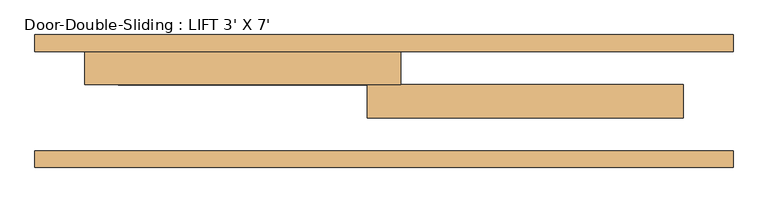
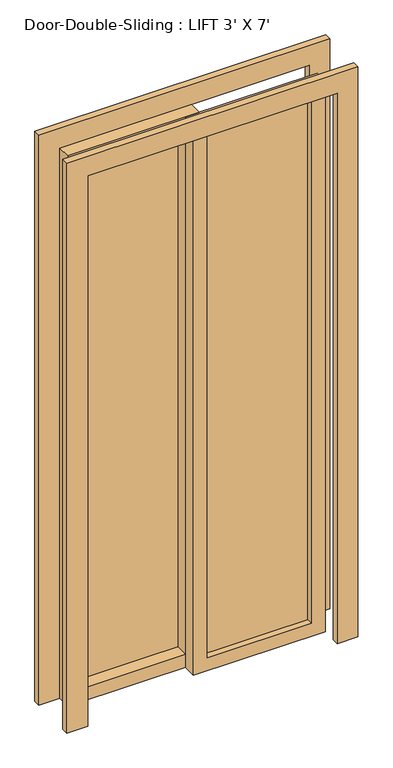
"""IFC4 building model written with IfcOpenShell, lengths in millimetres: door geometry, Door-Double-Sliding : LIFT 3' X 7'."""

from ifc_helpers import new_model, si_unit, frame, origin, place, context, project, spatial, polyline, outline, extrude, source, transform, mapped, element, save


def door_double_sliding_lift_3_x_7_7d4312a2(model_context):
    return source(origin(), model_context, "Body", "SweptSolid", [
        extrude(outline(polyline([(0.0, 533.4), (2209.8, 533.4), (2209.8, -533.4), (0.0, -533.4), (0.0, -457.2), (2133.6, -457.2), (2133.6, 457.2), (0.0, 457.2), (0.0, 533.4)])), frame((0.0, 203.2, 0.0), z_axis=(0.0, 1.0, 0.0), x_axis=(0.0, 0.0, 1.0)), (0.0, 0.0, 1.0), 25.4),
        extrude(outline(polyline([(0.0, -533.4), (0.0, -457.2), (2133.6, -457.2), (2133.6, 457.2), (0.0, 457.2), (0.0, 533.4), (2209.8, 533.4), (2209.8, -533.4), (0.0, -533.4)])), frame((0.0, 25.4, 0.0), z_axis=(0.0, 1.0, 0.0), x_axis=(0.0, 0.0, 1.0)), (0.0, 0.0, 1.0), 25.4),
        extrude(outline(polyline([(2133.6, 25.4), (2133.6, -457.2), (0.0, -457.2), (0.0, 25.4), (2133.6, 25.4)]), holes=[polyline([(2082.8, -25.4), (50.8, -25.4), (50.8, -406.4), (2082.8, -406.4), (2082.8, -25.4)])]), frame((0.0, 152.4, 0.0), z_axis=(0.0, 1.0, 0.0), x_axis=(0.0, 0.0, 1.0)), (0.0, 0.0, 1.0), 50.8),
        extrude(outline(polyline([(2133.6, -25.4), (0.0, -25.4), (0.0, 457.2), (2133.6, 457.2), (2133.6, -25.4)]), holes=[polyline([(2082.8, 25.4), (2082.8, 406.4), (50.8, 406.4), (50.8, 25.4), (2082.8, 25.4)])]), frame((0.0, 101.6, 0.0), z_axis=(0.0, 1.0, 0.0), x_axis=(0.0, 0.0, 1.0)), (0.0, 0.0, 1.0), 50.8),
        extrude(outline(polyline([(-25.4, 200.025), (-406.4, 200.025), (-406.4, 206.375), (-25.4, 206.375), (-25.4, 200.025)])), frame((0.0, 0.0, 50.8), z_axis=(0.0, 0.0, 1.0), x_axis=(1.0, 0.0, 0.0)), (0.0, 0.0, 1.0), 2032.0),
        extrude(outline(polyline([(25.4, 130.175), (406.4, 130.175), (406.4, 123.825), (25.4, 123.825), (25.4, 130.175)])), frame((0.0, 0.0, 50.8), z_axis=(0.0, 0.0, 1.0), x_axis=(1.0, 0.0, 0.0)), (0.0, 0.0, 1.0), 2032.0),
    ])


if __name__ == "__main__":
    model = new_model("IFC4")
    model_context = context("Model", 3, world=origin())
    ifc_project = project(units=[si_unit("LENGTHUNIT", "METRE", prefix="MILLI")], contexts=[model_context])
    site = spatial("IfcSite", under=ifc_project)
    building = spatial("IfcBuilding", under=site)
    placement = place(None, origin())
    door_double_sliding_lift_3_x_7_shape = door_double_sliding_lift_3_x_7_7d4312a2(model_context)
    element("IfcDoor", 1, ObjectType="Door-Double-Sliding : LIFT 3' X 7'", at=placement, inside=building, context=model_context, shape_type="MappedRepresentation", body=[
        mapped(door_double_sliding_lift_3_x_7_shape, transform((0.0, 0.0, 0.0), x_axis=(1.0, 0.0, 0.0), y_axis=(0.0, 1.0, 0.0), z_axis=(0.0, 0.0, 1.0))),
    ])
    save(model, "model.ifc")

# Revit data of these elements
# Type "Door-Double-Sliding : LIFT 3' X 7'"
#   Type Mark = "11"
#   Construction Type Id = "opn-d45"
#   Assembly Code = "C1020"
#   Analytic Construction = "Wood frame, double glass door "
#   Thickness = 0' - 2"
#   Thermal Resistance (R) = 1.8150 (h·ft²·°F)/BTU
#   Heat Transfer Coefficient (U) = 0.5510 BTU/(h·ft²·°F)
#   Height = 7' - 0"
#   Rail Width = 0' - 2"
#   Stiles = 0' - 2"
#   Trim Projection Ext = 0' - 1"
#   Trim Projection Int = 0' - 1"
#   Trim Width = 0' - 3"
#   Width = 3' - 0"
#   Define Thermal Properties by = 1
#   Glazing = Glass
#   Panel Material = Wood - Birch - Solid Stained Light Low Gloss
#   Trim Material = Paint - Sienna
#   Visual Light Transmittance = 0
#   Solar Heat Gain Coefficient = 0
#   Function = (empty or 0)
#   Wall Closure = (empty or 0)
# Element 1 (IfcDoor, "Door-Double-Sliding : LIFT 3' X 7'")
#   Materials on its faces: "Paint - Sienna", "Wood - Birch - Solid Stained Light Low Gloss", "Glass"
# Materials
#   "Glass": class "Glass", colour RGB 0 128 192, transparency 0.75, Description = "Soda Lime Glass", Cost = 0
#   "Wood - Birch - Solid Stained Light Low Gloss": class "Wood", colour RGB 210 159 95, transparency 0, Cost = 0
#   "Paint - Sienna": colour RGB 118 70 51, transparency 0, Cost = 0
